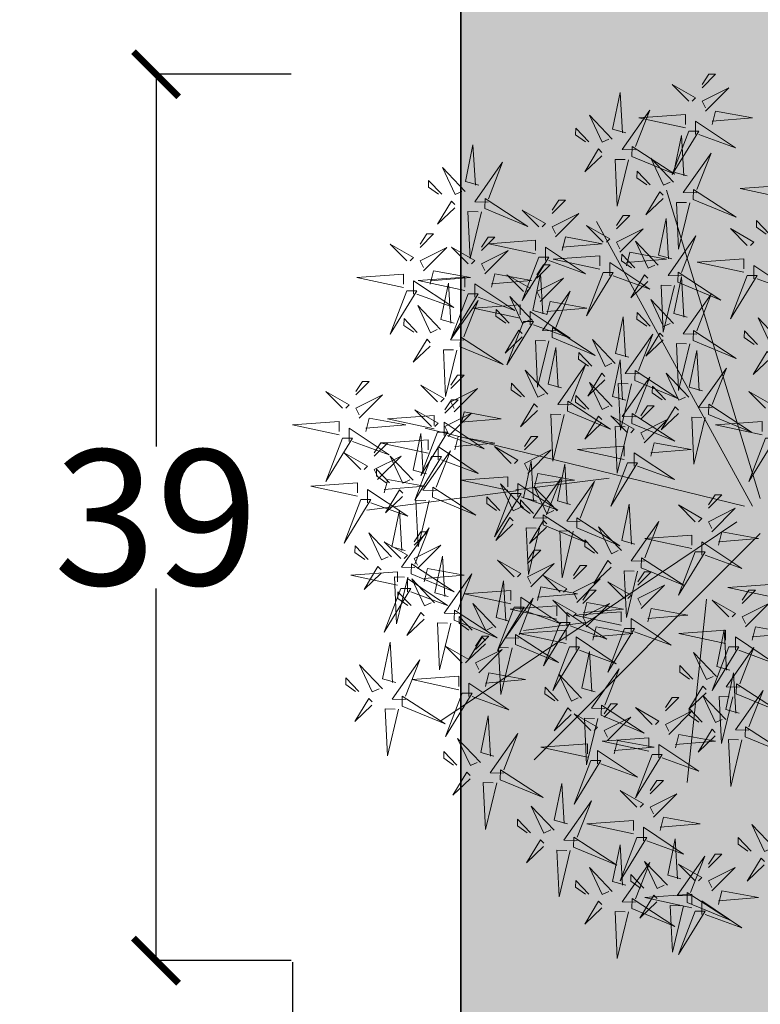
# Model space of a CAD drawing. Units: inches. Extents: x 1704 to 6393, y -157 to 1172.
# Tile 15 of 122: x 1879 to 1912, y 157 to 201. Entities that reach past the tile are written whole.
import ezdxf

# ---------------------------------------------------------------- set-up
doc = ezdxf.new("R2010")
doc.units = ezdxf.units.IN
doc.header["$MEASUREMENT"] = 0
for name, color, linetype, lineweight in [('A-ANNO-DIMS', 7, 'Continuous', 13), ('C-PROP', 7, 'Continuous', 35), ('L-shrub', 74, 'Continuous', 18)]:
    doc.layers.add(name, color=color, linetype=linetype, lineweight=lineweight)
doc.layers.add('L-PLNT-PATT', color=253, linetype='Continuous', lineweight=13, true_color=0x9abc8f)
doc.styles.get("Standard").update_dxf_attribs({"font": 'arial.ttf'})
doc.dimstyles.get("Standard").update_dxf_attribs({"dimtxt": 6, "dimasz": 2, "dimexe": 0.18, "dimexo": 0.0625, "dimgap": 0.09, "dimtad": 0, "dimtih": 1, "dimtoh": 1, "dimdec": 1, "dimzin": 0, "dimdsep": 46, "dimlunit": 3, "dimtxsty": 'Standard', "dimblk": 'ARCHTICK', "dimcen": 0.09, "dimadec": 0, "dimazin": 0, "dimtfac": 1, "dimtdec": 1, "dimtofl": 0, "dimtmove": 0, "dimatfit": 3, "dimfxl": 1, "dimtolj": 1, "dimtzin": 0, "dimarcsym": 0})

# ---------------------------------------------------------------- blocks, each defined once
blk = doc.blocks.new('shrub3')
for p, q in [((-11.38, -5.19), (-224.23, -69.78)), ((12.87, -5.19), (169.14, -161.27)), ((-5.99, -10.57), (-202.68, -118.21)), ((-5.99, -15.96), (-59.88, -236.62)), ((4.78, -21.34), (142.19, -225.85)), ((58.17, -42.16), (184.8, -55.61)), ((-17.27, -174.02), (-25.36, -109.43)), ((74.33, -125.58), (79.72, -168.64)), ((-16.77, -172.03), (-3.3, -276.98))]:
    blk.add_line(p, q)
for points in [[(-163.04, -9.56), (-172.27, -9.56), (-153.8, 18.11), (-163.04, -7.25)], [(86.56, -10.73), (77.32, -8.43), (81.94, 16.94), (84.25, -10.73)], [(153.14, -15.45), (165.42, 14.26), (146.23, -15.28), (153.14, -15.45)], [(-218.53, 13.17), (-225.46, -19.11), (-227.77, 13.17), (-220.84, 13.17)], [(-119.49, 9.1), (-136.03, -6.65), (-117.36, 2.12), (-119.55, 6.79)], [(123.46, -21.81), (135.74, 7.91), (116.55, -21.63), (123.46, -21.81)], [(-193.91, 1.36), (-203.36, -7.64), (-198.75, -7.76), (-193.97, -0.95)], [(-108.14, 1.89), (-96.9, -9.94), (-112.81, -0.3), (-110.44, 1.95)], [(-73.76, -1.46), (-85.3, -12.99), (-76.07, 3.15), (-73.76, 0.84)], [(-52.98, -1.46), (-22.97, -12.99), (-52.98, 5.45), (-52.98, -1.46)], [(57.07, 4.7), (50.14, -27.58), (47.83, 4.7), (54.76, 4.7)], [(77.32, -15.34), (61.16, 0.8), (70.4, -17.65), (75.02, -15.34)], [(93.49, -22.26), (84.25, -22.26), (102.72, 5.41), (93.49, -19.96)], [(230.31, 4.87), (213.77, -10.89), (232.44, -2.12), (230.25, 2.56)], [(-55.29, -3.77), (-62.22, -36.05), (-64.53, -3.77), (-57.6, -3.77)], [(20.84, -34.02), (11.6, -31.72), (16.22, -6.36), (18.53, -34.02)], [(148.59, -13.03), (148.36, -22.26), (121.16, -3.11), (146.29, -12.97)], [(241.66, -2.35), (252.9, -14.18), (237, -4.54), (239.36, -2.29)], [(268.88, -34.02), (259.65, -31.72), (264.26, -6.36), (266.57, -34.02)], [(-269.6, -38.26), (-278.84, -35.95), (-274.22, -10.59), (-271.91, -38.26)], [(-186.12, -14.17), (-197.67, -25.7), (-188.43, -9.56), (-186.12, -11.86)], [(-165.34, -14.17), (-135.33, -25.7), (-165.34, -7.25), (-165.34, -14.17)], [(-117.59, -7.11), (-127.04, -16.11), (-122.43, -16.23), (-117.65, -9.42)], [(-69.46, -40.86), (-57.18, -11.15), (-76.37, -40.69), (-69.46, -40.86)], [(61.16, -17.65), (51.93, -8.43), (51.93, -13.04), (58.86, -17.65)], [(118.91, -19.38), (118.68, -28.61), (91.48, -9.46), (116.61, -19.33)], [(232.21, -11.35), (222.76, -20.35), (227.37, -20.46), (232.16, -13.66)], [(-167.65, -16.47), (-174.58, -48.76), (-176.89, -16.47), (-169.96, -16.47)], [(27.76, -45.55), (18.53, -45.55), (37, -17.88), (27.76, -43.25)], [(91.18, -26.87), (121.19, -38.4), (91.18, -19.96), (91.18, -26.87)], [(136.89, -19.67), (134.36, -28.84), (109.12, -23.59), (136.84, -21.97)], [(155.39, -17.82), (187.49, -25.55), (155.16, -27.05), (155.33, -20.13)], [(275.81, -45.55), (266.57, -45.55), (285.04, -17.88), (275.81, -43.25)], [(-278.84, -42.87), (-295, -26.73), (-285.76, -45.18), (-281.15, -42.87)], [(-262.68, -49.79), (-271.91, -49.79), (-253.44, -22.12), (-262.68, -47.48)], [(-217.86, -51.45), (-205.58, -21.74), (-224.77, -51.28), (-217.86, -51.45)], [(-120.34, -51.45), (-108.06, -21.74), (-127.25, -51.28), (-120.34, -51.45)], [(11.6, -38.64), (-4.56, -22.5), (4.68, -40.94), (9.3, -38.64)], [(70.4, -26.87), (58.86, -38.4), (68.09, -22.26), (70.4, -24.57)], [(107.21, -26.02), (104.68, -35.19), (79.44, -29.94), (107.16, -28.33)], [(125.71, -24.17), (157.81, -31.9), (125.48, -33.4), (125.65, -26.48)], [(259.65, -38.64), (243.49, -22.5), (252.72, -40.94), (257.34, -38.64)], [(267.62, -55.68), (279.9, -25.97), (260.71, -55.51), (267.62, -55.68)], [(-160.62, -62.04), (-148.34, -32.32), (-167.53, -61.86), (-160.62, -62.04)], [(-74.01, -38.44), (-74.24, -47.67), (-101.44, -28.52), (-76.31, -38.38)], [(-4.56, -40.94), (-13.79, -31.72), (-13.79, -36.33), (-6.86, -40.94)], [(88.87, -29.18), (81.94, -61.46), (79.63, -29.18), (86.56, -29.18)], [(141.27, -29.01), (124.73, -44.76), (143.4, -35.99), (141.21, -31.32)], [(243.49, -40.94), (234.25, -31.72), (234.25, -36.33), (241.18, -40.94)], [(-295, -45.18), (-304.23, -35.95), (-304.23, -40.56), (-297.31, -45.18)], [(-222.41, -49.03), (-222.64, -58.26), (-249.84, -39.1), (-224.72, -48.97)], [(-124.89, -49.03), (-125.12, -58.26), (-152.32, -39.1), (-127.2, -48.97)], [(111.59, -35.37), (95.05, -51.12), (113.72, -42.35), (111.53, -37.67)], [(152.62, -36.23), (163.86, -48.05), (147.96, -38.42), (150.32, -36.17)], [(160.76, -63.67), (151.53, -61.36), (156.14, -36), (158.45, -63.67)], [(-264.99, -54.4), (-234.97, -65.93), (-264.99, -47.48), (-264.99, -54.4)], [(-85.71, -45.07), (-88.24, -54.25), (-113.48, -49), (-85.77, -47.38)], [(-67.21, -43.23), (-35.11, -50.96), (-67.44, -52.46), (-67.27, -45.54)], [(4.68, -50.16), (-6.86, -61.69), (2.37, -45.55), (4.68, -47.86)], [(25.46, -50.16), (55.47, -61.69), (25.46, -43.25), (25.46, -50.16)], [(122.94, -42.58), (134.18, -54.41), (118.28, -44.77), (120.64, -42.52)], [(143.17, -45.23), (133.72, -54.23), (138.33, -54.34), (143.12, -47.53)], [(167.69, -75.2), (158.45, -75.2), (176.92, -47.53), (167.69, -72.89)], [(218, -74.25), (208.77, -71.95), (213.38, -46.59), (215.69, -74.25)], [(263.07, -53.26), (262.84, -62.49), (235.64, -43.34), (260.77, -53.2)], [(252.72, -50.16), (241.18, -61.69), (250.41, -45.55), (252.72, -47.86)], [(273.5, -50.16), (303.51, -61.69), (273.5, -43.25), (273.5, -50.16)], [(-285.76, -54.4), (-297.31, -65.93), (-288.07, -49.79), (-285.76, -52.09)], [(-215.61, -53.82), (-183.51, -61.55), (-215.84, -63.05), (-215.67, -56.12)], [(-165.17, -59.61), (-165.4, -68.85), (-192.6, -49.69), (-167.48, -59.56)], [(-118.09, -53.82), (-85.99, -61.55), (-118.32, -63.05), (-118.15, -56.12)], [(-40.64, -80.61), (-49.88, -78.3), (-45.26, -52.94), (-42.95, -80.61)], [(23.15, -52.47), (16.22, -84.75), (13.91, -52.47), (20.84, -52.47)], [(113.49, -51.58), (104.04, -60.58), (108.65, -60.69), (113.43, -53.89)], [(151.53, -68.28), (135.37, -52.14), (144.6, -70.59), (149.22, -68.28)], [(271.19, -52.47), (264.26, -84.75), (261.95, -52.47), (268.88, -52.47)], [(-267.29, -56.71), (-274.22, -88.99), (-276.53, -56.71), (-269.6, -56.71)], [(-234.11, -55.66), (-236.65, -64.84), (-261.89, -59.59), (-234.17, -57.97)], [(-136.59, -55.66), (-139.12, -64.84), (-164.36, -59.59), (-136.65, -57.97)], [(-81.33, -54.42), (-97.87, -70.17), (-79.2, -61.4), (-81.39, -56.73)], [(36.54, -87.45), (48.82, -57.73), (29.63, -87.27), (36.54, -87.45)], [(73.84, -82.72), (64.6, -80.42), (69.22, -55.06), (71.53, -82.72)], [(224.93, -85.78), (215.69, -85.78), (234.16, -58.11), (224.93, -83.48)], [(251.37, -59.9), (248.84, -69.07), (223.6, -63.82), (251.32, -62.2)], [(269.87, -58.05), (301.97, -65.78), (269.64, -67.28), (269.81, -60.36)], [(-247.54, -93.8), (-235.26, -64.08), (-254.45, -93.62), (-247.54, -93.8)], [(-229.73, -65.01), (-246.27, -80.76), (-227.6, -71.99), (-229.79, -67.32)], [(-176.87, -66.25), (-179.4, -75.42), (-204.64, -70.17), (-176.93, -68.56)], [(-158.37, -64.4), (-126.27, -72.13), (-158.6, -73.63), (-158.43, -66.71)], [(-132.21, -65.01), (-148.75, -80.76), (-130.08, -71.99), (-132.27, -67.32)], [(-92.78, -91.68), (-80.5, -61.97), (-99.69, -91.51), (-92.78, -91.68)], [(-69.98, -61.63), (-58.74, -73.46), (-74.65, -63.83), (-72.28, -61.58)], [(-63.1, -93.8), (-50.82, -64.08), (-70.01, -93.62), (-63.1, -93.8)], [(-33.72, -92.14), (-42.95, -92.14), (-24.48, -64.47), (-33.72, -89.83)], [(80.77, -94.25), (71.53, -94.25), (90, -66.58), (80.77, -91.95)], [(135.37, -70.59), (126.13, -61.36), (126.13, -65.97), (133.06, -70.59)], [(208.77, -78.87), (192.61, -62.73), (201.84, -81.17), (206.46, -78.87)], [(271.86, -93.8), (284.14, -64.08), (264.95, -93.62), (271.86, -93.8)], [(-218.38, -72.22), (-207.14, -84.05), (-223.05, -74.41), (-220.68, -72.16)], [(-172.08, -97.55), (-181.32, -95.24), (-176.7, -69.88), (-174.39, -97.55)], [(-120.86, -72.22), (-109.62, -84.05), (-125.53, -74.41), (-123.16, -72.16)], [(-79.43, -70.63), (-88.88, -79.64), (-84.27, -79.75), (-79.49, -72.94)], [(-49.88, -85.22), (-66.04, -69.08), (-56.8, -87.52), (-52.18, -85.22)], [(64.6, -87.34), (48.44, -71.2), (57.68, -89.64), (62.3, -87.34)], [(165.38, -79.81), (195.39, -91.34), (165.38, -72.89), (165.38, -79.81)], [(192.61, -81.17), (183.37, -71.95), (183.37, -76.56), (190.3, -81.17)], [(255.75, -69.24), (239.21, -85), (257.88, -76.23), (255.7, -71.55)], [(-252.09, -91.37), (-252.32, -100.61), (-279.52, -81.45), (-254.4, -91.32)], [(-227.83, -81.22), (-237.28, -90.22), (-232.67, -90.34), (-227.89, -83.53)], [(-172.49, -75.6), (-189.03, -91.35), (-170.36, -82.58), (-172.55, -77.9)], [(-165.16, -109.08), (-174.39, -109.08), (-155.92, -81.41), (-165.16, -106.77)], [(-130.31, -81.22), (-139.76, -90.22), (-135.15, -90.34), (-130.37, -83.53)], [(-97.33, -89.26), (-97.56, -98.49), (-124.76, -79.33), (-99.63, -89.2)], [(-67.65, -91.37), (-67.88, -100.61), (-95.08, -81.45), (-69.95, -91.32)], [(-66.04, -87.52), (-75.27, -78.3), (-75.27, -82.91), (-68.34, -87.52)], [(31.99, -85.02), (31.76, -94.25), (4.56, -75.1), (29.69, -84.96)], [(48.44, -89.64), (39.21, -80.42), (39.21, -85.03), (46.14, -89.64)], [(144.6, -79.81), (133.06, -91.34), (142.29, -75.2), (144.6, -77.5)], [(165, -106.02), (155.77, -103.71), (160.38, -78.35), (162.69, -106.02)], [(267.31, -91.37), (267.08, -100.61), (239.88, -81.45), (265.01, -91.32)], [(267.1, -76.46), (278.34, -88.28), (262.44, -78.65), (264.8, -76.4)], [(-181.32, -102.16), (-197.48, -86.02), (-188.24, -104.46), (-183.63, -102.16)], [(-161.14, -82.81), (-149.9, -94.64), (-165.81, -85), (-163.44, -82.75)], [(138.3, -114.97), (150.58, -85.26), (131.39, -114.8), (138.3, -114.97)], [(163.07, -82.11), (156.14, -114.39), (153.83, -82.11), (160.76, -82.11)], [(201.84, -90.4), (190.3, -101.92), (199.53, -85.78), (201.84, -88.09)], [(222.62, -90.4), (252.63, -101.92), (222.62, -83.48), (222.62, -90.4)], [(257.65, -85.46), (248.2, -94.46), (252.81, -94.57), (257.6, -87.76)], [(-170.59, -91.81), (-180.04, -100.81), (-175.43, -100.93), (-170.65, -94.12)], [(-90.53, -94.05), (-58.43, -101.78), (-90.76, -103.28), (-90.59, -96.35)], [(-56.8, -96.75), (-68.34, -108.28), (-59.11, -92.14), (-56.8, -94.44)], [(-36.02, -96.75), (-6.01, -108.28), (-36.02, -89.83), (-36.02, -96.75)], [(20.29, -91.66), (17.76, -100.83), (-7.48, -95.58), (20.23, -93.97)], [(38.79, -89.81), (70.89, -97.54), (38.56, -99.04), (38.73, -92.12)], [(57.68, -98.86), (46.14, -110.39), (55.37, -94.25), (57.68, -96.56)], [(86.56, -120.84), (77.32, -118.53), (81.94, -93.17), (84.25, -120.84)], [(78.46, -98.86), (108.47, -110.39), (78.46, -91.95), (78.46, -98.86)], [(155.77, -110.63), (139.61, -94.49), (148.84, -112.93), (153.46, -110.63)], [(171.93, -117.54), (162.69, -117.54), (181.16, -89.88), (171.93, -115.24)], [(220.31, -92.7), (213.38, -124.98), (211.07, -92.7), (218, -92.7)], [(-263.79, -98.01), (-266.33, -107.18), (-291.57, -101.93), (-263.85, -100.32)], [(-245.29, -96.16), (-213.19, -103.89), (-245.52, -105.4), (-245.35, -98.47)], [(-197.48, -104.46), (-206.71, -95.24), (-206.71, -99.85), (-199.79, -104.46)], [(-109.03, -95.89), (-111.56, -105.07), (-136.8, -99.82), (-109.09, -98.2)], [(-79.35, -98.01), (-81.88, -107.18), (-107.12, -101.93), (-79.41, -100.32)], [(-60.85, -96.16), (-28.75, -103.89), (-61.08, -105.4), (-60.91, -98.47)], [(-38.33, -99.05), (-45.26, -131.33), (-47.57, -99.05), (-40.64, -99.05)], [(24.67, -101), (8.13, -116.76), (26.8, -107.99), (24.61, -103.31)], [(69.6, -127.19), (60.36, -124.88), (64.98, -99.52), (67.29, -127.19)], [(76.15, -101.17), (69.22, -133.45), (66.91, -101.17), (73.84, -101.17)], [(255.61, -98.01), (253.08, -107.18), (227.84, -101.93), (255.56, -100.32)], [(274.11, -96.16), (306.21, -103.89), (273.88, -105.4), (274.05, -98.47)], [(-259.41, -107.36), (-275.95, -123.11), (-257.28, -114.34), (-259.47, -109.66)], [(-167.46, -113.69), (-137.45, -125.22), (-167.46, -106.77), (-167.46, -113.69)], [(-104.65, -105.24), (-121.19, -120.99), (-102.52, -112.22), (-104.71, -107.55)], [(-74.97, -107.36), (-91.51, -123.11), (-72.84, -114.34), (-75.03, -109.66)], [(-71.58, -138.26), (-59.3, -108.55), (-78.49, -138.09), (-71.58, -138.26)], [(8.98, -131.91), (21.26, -102.2), (2.07, -131.74), (8.98, -131.91)], [(36.02, -108.22), (47.26, -120.04), (31.36, -110.41), (33.72, -108.16)], [(93.49, -132.37), (84.25, -132.37), (102.72, -104.7), (93.49, -130.06)], [(133.75, -112.55), (133.52, -121.78), (106.32, -102.62), (131.45, -112.49)], [(139.61, -112.93), (130.37, -103.71), (130.37, -108.32), (137.3, -112.93)], [(229.46, -134.03), (241.74, -104.31), (222.55, -133.86), (229.46, -134.03)], [(259.99, -107.36), (243.45, -123.11), (262.12, -114.34), (259.94, -109.66)], [(-248.06, -114.57), (-236.82, -126.4), (-252.73, -116.76), (-250.36, -114.51)], [(-188.24, -113.69), (-199.79, -125.22), (-190.55, -109.08), (-188.24, -111.38)], [(-182.68, -142.01), (-191.92, -139.71), (-187.3, -114.34), (-184.99, -142.01)], [(-93.3, -112.45), (-82.06, -124.28), (-97.97, -114.64), (-95.6, -112.39)], [(-63.62, -114.57), (-52.38, -126.4), (-68.29, -116.76), (-65.92, -114.51)], [(77.32, -125.45), (61.16, -109.31), (70.4, -127.75), (75.02, -125.45)], [(76.53, -138.72), (67.29, -138.72), (85.76, -111.05), (76.53, -136.41)], [(169.62, -122.16), (199.63, -133.69), (169.62, -115.24), (169.62, -122.16)], [(271.34, -114.57), (282.58, -126.4), (266.68, -116.76), (269.04, -114.51)], [(-169.77, -115.99), (-176.7, -148.27), (-179.01, -115.99), (-172.08, -115.99)], [(-122.46, -148.85), (-110.18, -119.14), (-129.37, -148.68), (-122.46, -148.85)], [(-102.75, -121.45), (-112.2, -130.45), (-107.59, -130.57), (-102.81, -123.76)], [(4.43, -129.49), (4.2, -138.72), (-23, -119.56), (2.13, -129.43)], [(26.57, -117.22), (17.12, -126.22), (21.73, -126.33), (26.51, -119.53)], [(60.36, -131.8), (44.2, -115.66), (53.44, -134.11), (58.06, -131.8)], [(61.16, -127.75), (51.93, -118.53), (51.93, -123.14), (58.86, -127.75)], [(122.05, -119.18), (119.52, -128.36), (94.28, -123.11), (122, -121.49)], [(148.84, -122.16), (137.3, -133.69), (146.53, -117.54), (148.84, -119.85)], [(140.55, -117.34), (172.65, -125.07), (140.32, -126.57), (140.49, -119.65)], [(224.91, -131.61), (224.68, -140.84), (197.48, -121.68), (222.61, -131.55)], [(-257.51, -123.57), (-266.96, -132.57), (-262.35, -132.69), (-257.57, -125.88)], [(-175.76, -153.54), (-184.99, -153.54), (-166.52, -125.87), (-175.76, -151.23)], [(-138.16, -152.6), (-147.4, -150.29), (-142.78, -124.93), (-140.47, -152.6)], [(-76.13, -135.84), (-76.36, -145.07), (-103.56, -125.92), (-78.43, -135.78)], [(-73.07, -123.57), (-82.52, -132.57), (-77.91, -132.69), (-73.13, -125.88)], [(6.86, -155.2), (19.14, -125.49), (-0.05, -155.03), (6.86, -155.2)], [(44.2, -134.11), (34.97, -124.88), (34.97, -129.5), (41.9, -134.11)], [(126.43, -128.53), (109.89, -144.28), (128.56, -135.51), (126.37, -130.84)], [(167.31, -124.46), (160.38, -156.74), (158.07, -124.46), (165, -124.46)], [(261.89, -123.57), (252.44, -132.57), (257.05, -132.69), (261.84, -125.88)], [(-191.92, -146.62), (-208.08, -130.48), (-198.84, -148.93), (-194.23, -146.62)], [(-19.44, -161.07), (-28.68, -158.76), (-24.06, -133.4), (-21.75, -161.07)], [(11.23, -134.28), (43.33, -142.01), (11, -143.51), (11.17, -136.58)], [(59, -158.95), (49.76, -156.64), (54.38, -131.28), (56.69, -158.95)], [(70.4, -136.98), (58.86, -148.51), (68.09, -132.37), (70.4, -134.67)], [(91.18, -136.98), (121.19, -148.51), (91.18, -130.06), (91.18, -136.98)], [(137.78, -135.74), (149.02, -147.57), (133.12, -137.94), (135.48, -135.69)], [(-208.08, -148.93), (-217.31, -139.71), (-217.31, -144.32), (-210.39, -148.93)], [(-147.4, -157.21), (-163.56, -141.07), (-154.32, -159.52), (-149.71, -157.21)], [(-127.01, -146.43), (-127.24, -155.66), (-154.44, -136.5), (-129.32, -146.37)], [(-131.24, -164.13), (-140.47, -164.13), (-122, -136.46), (-131.24, -161.82)], [(-87.83, -142.48), (-90.36, -151.65), (-115.6, -146.4), (-87.89, -144.78)], [(-69.33, -140.63), (-37.23, -148.36), (-69.56, -149.86), (-69.39, -142.94)], [(-7.27, -136.12), (-9.8, -145.3), (-35.04, -140.05), (-7.33, -138.43)], [(53.44, -143.33), (41.9, -154.86), (51.13, -138.72), (53.44, -141.02)], [(74.22, -143.33), (104.23, -154.86), (74.22, -136.41), (74.22, -143.33)], [(88.87, -139.28), (81.94, -171.56), (79.63, -139.28), (86.56, -139.28)], [(213.21, -138.24), (210.68, -147.41), (185.44, -142.16), (213.16, -140.55)], [(231.71, -136.39), (263.81, -144.13), (231.48, -145.63), (231.65, -138.7)], [(-28.68, -165.68), (-44.84, -149.54), (-35.6, -167.99), (-30.98, -165.68)], [(2.31, -152.78), (2.08, -162.01), (-25.12, -142.86), (0.01, -152.72)], [(-12.52, -172.6), (-21.75, -172.6), (-3.28, -144.93), (-12.52, -170.29)], [(-2.89, -145.47), (-19.43, -161.22), (-0.76, -152.45), (-2.95, -147.78)], [(49.76, -163.56), (33.6, -147.42), (42.84, -165.87), (47.46, -163.56)], [(65.93, -170.48), (56.69, -170.48), (75.16, -142.81), (65.93, -168.17)], [(71.91, -145.64), (64.98, -177.92), (62.67, -145.64), (69.6, -145.64)], [(89.54, -174.26), (101.82, -144.54), (82.63, -174.09), (89.54, -174.26)], [(128.33, -144.74), (118.88, -153.74), (123.49, -153.86), (128.27, -147.05)], [(217.59, -147.59), (201.05, -163.34), (219.72, -154.57), (217.53, -149.9)], [(-198.84, -158.15), (-210.39, -169.68), (-201.15, -153.54), (-198.84, -155.85)], [(-178.06, -158.15), (-148.05, -169.68), (-178.06, -151.23), (-178.06, -158.15)], [(-163.56, -159.52), (-172.79, -150.29), (-172.79, -154.9), (-165.87, -159.52)], [(-138.71, -153.06), (-141.24, -162.24), (-166.48, -156.99), (-138.77, -155.37)], [(-120.21, -151.22), (-88.11, -158.95), (-120.44, -160.45), (-120.27, -153.52)], [(-83.45, -151.82), (-99.99, -167.57), (-81.32, -158.8), (-83.51, -154.13)], [(8.46, -152.68), (19.7, -164.51), (3.8, -154.87), (6.16, -152.62)], [(182.82, -184.85), (195.1, -155.13), (175.91, -184.67), (182.82, -184.85)], [(228.94, -154.8), (240.18, -166.63), (224.28, -156.99), (226.64, -154.74)], [(-180.37, -160.46), (-187.3, -192.74), (-189.61, -160.46), (-182.68, -160.46)], [(-157.24, -190.71), (-166.48, -188.41), (-161.86, -163.04), (-159.55, -190.71)], [(-134.33, -162.41), (-150.87, -178.16), (-132.2, -169.39), (-134.39, -164.72)], [(-133.54, -168.74), (-103.53, -180.27), (-133.54, -161.82), (-133.54, -168.74)], [(-72.1, -159.03), (-60.86, -170.86), (-76.77, -161.23), (-74.4, -158.98)], [(-44.84, -167.99), (-54.07, -158.76), (-54.07, -163.37), (-47.14, -167.99)], [(-9.39, -159.41), (-11.92, -168.59), (-37.16, -163.34), (-9.45, -161.72)], [(-0.99, -161.68), (-10.44, -170.68), (-5.83, -170.8), (-1.05, -163.99)], [(9.11, -157.57), (41.21, -165.3), (8.88, -166.8), (9.05, -159.88)], [(33.6, -165.87), (24.37, -156.64), (24.37, -161.26), (31.3, -165.87)], [(84.99, -171.84), (84.76, -181.07), (57.56, -161.91), (82.69, -171.78)], [(-211.5, -195.43), (-199.22, -165.72), (-218.41, -195.26), (-211.5, -195.43)], [(-154.32, -168.74), (-165.87, -180.27), (-156.63, -164.13), (-154.32, -166.43)], [(-122.98, -169.62), (-111.74, -181.45), (-127.65, -171.81), (-125.28, -169.56)], [(-81.55, -168.04), (-91, -177.04), (-86.39, -177.15), (-81.61, -170.34)], [(-5.01, -168.76), (-21.55, -184.51), (-2.88, -175.74), (-5.07, -171.07)], [(63.62, -175.09), (93.63, -186.62), (63.62, -168.17), (63.62, -175.09)], [(118.36, -194.95), (109.13, -192.64), (113.74, -167.28), (116.05, -194.95)], [(219.49, -163.8), (210.04, -172.8), (214.65, -172.92), (219.44, -166.11)], [(-150.32, -202.24), (-159.55, -202.24), (-141.08, -174.57), (-150.32, -199.93)], [(-135.85, -171.04), (-142.78, -203.33), (-145.09, -171.04), (-138.16, -171.04)], [(-35.6, -177.21), (-47.14, -188.74), (-37.91, -172.6), (-35.6, -174.9)], [(-14.82, -177.21), (15.19, -188.74), (-14.82, -170.29), (-14.82, -177.21)], [(6.34, -175.97), (17.58, -187.8), (1.68, -178.17), (4.04, -175.92)], [(42.84, -175.09), (31.3, -186.62), (40.53, -170.48), (42.84, -172.79)], [(91.79, -176.62), (123.89, -184.36), (91.56, -185.86), (91.73, -178.93)], [(178.27, -182.42), (178.04, -191.65), (150.84, -172.5), (175.97, -182.36)], [(-216.05, -193.01), (-216.28, -202.24), (-243.48, -183.09), (-218.36, -192.95)], [(-166.48, -195.32), (-182.64, -179.18), (-173.4, -197.63), (-168.79, -195.32)], [(-132.43, -178.62), (-141.88, -187.62), (-137.27, -187.74), (-132.49, -180.93)], [(-116.1, -212.37), (-103.82, -182.66), (-123.01, -212.2), (-116.1, -212.37)], [(-17.13, -179.51), (-24.06, -211.79), (-26.37, -179.51), (-19.44, -179.51)], [(73.29, -178.47), (70.76, -187.64), (45.52, -182.39), (73.23, -180.78)], [(61.31, -177.4), (54.38, -209.68), (52.07, -177.4), (59, -177.4)], [(109.13, -199.56), (92.96, -183.42), (102.2, -201.86), (106.82, -199.56)], [(125.29, -206.48), (116.05, -206.48), (134.52, -178.81), (125.29, -204.17)], [(-182.64, -197.63), (-191.87, -188.41), (-191.87, -193.02), (-184.95, -197.63)], [(-61.84, -211.89), (-71.08, -209.58), (-66.46, -184.22), (-64.15, -211.89)], [(-44.88, -216.12), (-54.12, -213.81), (-49.5, -188.45), (-47.19, -216.12)], [(-3.11, -184.97), (-12.56, -193.97), (-7.95, -194.09), (-3.17, -187.28)], [(77.67, -187.82), (61.13, -203.57), (79.8, -194.8), (77.61, -190.13)], [(72.58, -216.61), (84.86, -186.89), (65.67, -216.43), (72.58, -216.61)], [(166.57, -189.06), (164.04, -198.23), (138.8, -192.98), (166.52, -191.37)], [(185.07, -187.21), (217.17, -194.94), (184.84, -196.44), (185.01, -189.52)], [(-54.92, -223.41), (-64.15, -223.41), (-45.68, -195.75), (-54.92, -221.11)], [(92.96, -201.86), (83.73, -192.64), (83.73, -197.25), (90.66, -201.86)], [(89.02, -195.03), (100.26, -206.86), (84.36, -197.22), (86.72, -194.97)], [(-227.75, -199.64), (-230.29, -208.82), (-255.53, -203.57), (-227.81, -201.95)], [(-209.25, -197.8), (-177.15, -205.53), (-209.48, -207.03), (-209.31, -200.11)], [(-173.4, -206.85), (-184.95, -218.38), (-175.71, -202.24), (-173.4, -204.55)], [(-152.62, -206.85), (-122.61, -218.38), (-152.62, -199.93), (-152.62, -206.85)], [(-120.65, -209.95), (-120.88, -219.18), (-148.08, -200.02), (-122.96, -209.89)], [(-71.08, -216.5), (-87.24, -200.36), (-78, -218.8), (-73.38, -216.5)], [(-37.96, -227.65), (-47.19, -227.65), (-28.72, -199.98), (-37.96, -225.34)], [(-12.22, -231.43), (0.06, -201.71), (-19.13, -231.26), (-12.22, -231.43)], [(170.95, -198.4), (154.41, -214.16), (173.08, -205.39), (170.89, -200.71)], [(-223.37, -208.99), (-239.91, -224.74), (-221.24, -215.97), (-223.43, -211.3)], [(-159.36, -233.06), (-168.6, -230.75), (-163.98, -205.39), (-161.67, -233.06)], [(-154.93, -209.16), (-161.86, -241.44), (-164.17, -209.16), (-157.24, -209.16)], [(-87.24, -218.8), (-96.47, -209.58), (-96.47, -214.19), (-89.54, -218.8)], [(-54.12, -220.73), (-70.28, -204.59), (-61.04, -223.04), (-56.42, -220.73)], [(46.28, -237.29), (37.04, -234.99), (41.66, -209.63), (43.97, -237.29)], [(68.03, -214.18), (67.8, -223.42), (40.6, -204.26), (65.73, -214.13)], [(79.57, -204.03), (70.12, -213.03), (74.73, -213.15), (79.51, -206.34)], [(102.2, -211.09), (90.66, -222.62), (99.89, -206.48), (102.2, -208.78)], [(122.98, -211.09), (152.99, -222.62), (122.98, -204.17), (122.98, -211.09)], [(182.3, -205.62), (193.54, -217.44), (177.64, -207.81), (180, -205.56)], [(-212.02, -216.2), (-200.78, -228.03), (-216.69, -218.4), (-214.32, -216.15)], [(-152.44, -244.59), (-161.67, -244.59), (-143.2, -216.92), (-152.44, -242.28)], [(-132.35, -216.58), (-134.88, -225.76), (-160.12, -220.51), (-132.41, -218.89)], [(-113.85, -214.74), (-81.75, -222.47), (-114.08, -223.97), (-113.91, -217.05)], [(-70.28, -223.04), (-79.51, -213.81), (-79.51, -218.43), (-72.58, -223.04)], [(40.78, -246.25), (53.06, -216.54), (33.87, -246.08), (40.78, -246.25)], [(120.67, -213.39), (113.74, -245.67), (111.43, -213.39), (118.36, -213.39)], [(172.85, -214.62), (163.4, -223.62), (168.01, -223.73), (172.8, -216.93)], [(-168.6, -237.67), (-184.76, -221.53), (-175.52, -239.98), (-170.91, -237.67)], [(-78, -228.03), (-89.54, -239.55), (-80.31, -223.41), (-78, -225.72)], [(-57.22, -228.03), (-27.21, -239.55), (-57.22, -221.11), (-57.22, -228.03)], [(-16.77, -229.01), (-17, -238.24), (-44.2, -219.08), (-19.07, -228.95)], [(56.33, -220.82), (53.8, -229.99), (28.56, -224.74), (56.27, -223.13)], [(53.21, -248.82), (43.97, -248.82), (62.44, -221.15), (53.21, -246.52)], [(74.83, -218.97), (106.93, -226.7), (74.6, -228.2), (74.77, -221.28)], [(131.94, -252.6), (144.22, -222.89), (125.03, -252.43), (131.94, -252.6)], [(-221.47, -225.2), (-230.92, -234.21), (-226.31, -234.32), (-221.53, -227.51)], [(-184.76, -239.98), (-193.99, -230.75), (-193.99, -235.37), (-187.07, -239.98)], [(-127.97, -225.93), (-144.51, -241.68), (-125.84, -232.91), (-128.03, -228.24)], [(-61.04, -232.26), (-72.58, -243.79), (-63.35, -227.65), (-61.04, -229.95)], [(-59.53, -230.33), (-66.46, -262.61), (-68.77, -230.33), (-61.84, -230.33)], [(-40.26, -232.26), (-10.25, -243.79), (-40.26, -225.34), (-40.26, -232.26)], [(37.04, -241.91), (20.88, -225.77), (30.12, -244.21), (34.74, -241.91)], [(60.71, -230.17), (44.17, -245.92), (62.84, -237.15), (60.65, -232.47)], [(-116.62, -233.14), (-105.38, -244.97), (-121.29, -235.34), (-118.92, -233.09)], [(-28.47, -235.64), (-31, -244.81), (-56.24, -239.56), (-28.53, -237.95)], [(-42.57, -234.57), (-49.5, -266.85), (-51.81, -234.57), (-44.88, -234.57)], [(-15.2, -264.82), (-24.44, -262.51), (-19.82, -237.15), (-17.51, -264.82)], [(-9.97, -233.79), (22.13, -241.53), (-10.2, -243.03), (-10.03, -236.1)], [(36.23, -243.83), (36, -253.06), (8.8, -233.9), (33.93, -243.77)], [(20.88, -244.21), (11.65, -234.99), (11.65, -239.6), (18.58, -244.21)], [(72.06, -237.38), (83.3, -249.21), (67.4, -239.57), (69.76, -237.32)], [(-175.52, -249.2), (-187.07, -260.73), (-177.83, -244.59), (-175.52, -246.89)], [(-154.74, -249.2), (-124.73, -260.73), (-154.74, -242.28), (-154.74, -249.2)], [(-126.07, -242.14), (-135.52, -251.14), (-130.91, -251.26), (-126.13, -244.45)], [(127.39, -250.18), (127.16, -259.41), (99.96, -240.26), (125.09, -250.12)], [(-157.05, -251.51), (-163.98, -283.79), (-166.29, -251.51), (-159.36, -251.51)], [(-57.6, -277.52), (-66.84, -275.22), (-62.22, -249.86), (-59.91, -277.52)], [(-24.09, -244.99), (-40.63, -260.74), (-21.96, -251.97), (-24.15, -247.3)], [(-8.28, -276.35), (-17.51, -276.35), (0.96, -248.68), (-8.28, -274.04)], [(24.53, -250.46), (22, -259.64), (-3.24, -254.39), (24.47, -252.77)], [(30.12, -253.43), (18.58, -264.96), (27.81, -248.82), (30.12, -251.13)], [(43.03, -248.62), (75.13, -256.35), (42.8, -257.85), (42.97, -250.92)], [(50.9, -253.43), (80.91, -264.96), (50.9, -246.52), (50.9, -253.43)], [(62.61, -246.38), (53.16, -255.38), (57.77, -255.49), (62.55, -248.69)], [(-24.44, -269.43), (-40.6, -253.29), (-31.36, -271.74), (-26.74, -269.43)], [(-12.74, -252.2), (-1.5, -264.03), (-17.4, -254.39), (-15.04, -252.14)], [(48.59, -255.74), (41.66, -288.02), (39.35, -255.74), (46.28, -255.74)], [(115.69, -256.81), (113.16, -265.99), (87.92, -260.74), (115.64, -259.12)], [(134.19, -254.97), (166.29, -262.7), (133.96, -264.2), (134.13, -257.28)], [(-50.68, -289.05), (-59.91, -289.05), (-41.44, -261.38), (-50.68, -286.75)], [(-40.6, -271.74), (-49.83, -262.51), (-49.83, -267.13), (-42.9, -271.74)], [(-22.19, -261.2), (-31.64, -270.2), (-27.03, -270.32), (-22.25, -263.51)], [(28.91, -259.81), (12.37, -275.56), (31.04, -266.79), (28.85, -262.12)], [(-66.84, -282.14), (-83, -266), (-73.76, -284.44), (-69.14, -282.14)], [(40.26, -267.02), (51.5, -278.85), (35.6, -269.21), (37.96, -266.96)], [(120.07, -266.16), (103.53, -281.91), (122.2, -273.14), (120.01, -268.47)], [(-83, -284.44), (-92.23, -275.22), (-92.23, -279.83), (-85.3, -284.44)], [(-31.36, -280.96), (-42.9, -292.49), (-33.67, -276.35), (-31.36, -278.65)], [(-10.58, -280.96), (19.43, -292.49), (-10.58, -274.04), (-10.58, -280.96)], [(30.81, -276.02), (21.36, -285.02), (25.97, -285.14), (30.75, -278.33)], [(131.42, -273.37), (142.66, -285.2), (126.76, -275.57), (129.12, -273.32)], [(-12.89, -283.27), (-19.82, -315.55), (-22.13, -283.27), (-15.2, -283.27)], [(121.97, -282.37), (112.52, -291.38), (117.13, -291.49), (121.91, -284.68)], [(-73.76, -293.67), (-85.3, -305.19), (-76.07, -289.05), (-73.76, -291.36)], [(-52.98, -293.67), (-22.97, -305.19), (-52.98, -286.75), (-52.98, -293.67)], [(-55.29, -295.97), (-62.22, -328.25), (-64.53, -295.97), (-57.6, -295.97)]]:
    blk.add_lwpolyline(points)
blk = doc.blocks.new('_ArchTick')
at = {"color": 0, "linetype": 'ByBlock', "const_width": 0.15}
blk.add_lwpolyline([(-0.5, -0.5), (0.5, 0.5)], dxfattribs=at)
blk = doc.blocks.new('*D74')
at = {"layer": 'A-ANNO-DIMS', "color": 0, "lineweight": -2, "transparency": 16777216}
for p, q in [((1890.878, 159.062), (1890.878, 152.884)), ((1931.278, 159.062), (1931.278, 152.884)), ((1890.878, 153.064), (1888.878, 153.064)), ((1931.278, 153.064), (1933.278, 153.064))]:
    blk.add_line(p, q, dxfattribs=at)
at = {"layer": 'Defpoints', "color": 0, "lineweight": -3, "transparency": 16777216}
for p in [(1890.878, 159.124), (1931.278, 159.124), (1931.278, 153.064)]:
    blk.add_point(p, dxfattribs=at)
at = {"layer": 'A-ANNO-DIMS', "color": 0, "lineweight": -2, "transparency": 16777216, "xscale": 2, "yscale": 2, "zscale": 2}
blk.add_blockref('_ArchTick', (1890.878, 153.064), dxfattribs=at)
at = {"layer": 'A-ANNO-DIMS', "color": 0, "lineweight": -2, "transparency": 16777216, "xscale": 2, "yscale": 2, "zscale": 2, "rotation": 180}
blk.add_blockref('_ArchTick', (1931.278, 153.064), dxfattribs=at)
at = {"layer": 'A-ANNO-DIMS', "color": 0, "transparency": 16777216, "insert": (1911.078, 153.064), "char_height": 6, "attachment_point": 5}
blk.add_mtext('\\A1;SHRUB 40', dxfattribs=at)
blk = doc.blocks.new('*D75')
at = {"layer": 'A-ANNO-DIMS', "color": 0, "lineweight": -2, "transparency": 16777216}
for p, q in [((1890.815, 198.475), (1884.637, 198.475)), ((1884.817, 198.475), (1884.817, 181.955)), ((1884.817, 159.124), (1884.817, 175.644)), ((1890.815, 159.124), (1884.637, 159.124))]:
    blk.add_line(p, q, dxfattribs=at)
at = {"layer": 'Defpoints', "color": 0, "lineweight": -3, "transparency": 16777216}
for p in [(1890.878, 198.475), (1884.817, 159.124), (1890.878, 159.124)]:
    blk.add_point(p, dxfattribs=at)
at = {"layer": 'A-ANNO-DIMS', "color": 0, "lineweight": -2, "transparency": 16777216, "xscale": 2, "yscale": 2, "zscale": 2}
for p, rotation in [((1884.817, 198.475), 90), ((1884.817, 159.124), 270)]:
    blk.add_blockref('_ArchTick', p, dxfattribs=dict(at, rotation=rotation))
at = {"layer": 'A-ANNO-DIMS', "color": 0, "transparency": 16777216, "insert": (1884.817, 178.8), "char_height": 6, "attachment_point": 5}
blk.add_mtext('\\A1;39', dxfattribs=at)
blk = doc.blocks.new('*D93')
at = {"layer": 'A-ANNO-DIMS', "color": 0, "lineweight": -2, "transparency": 16777216}
for p, q in [((2605.286, 895.213), (1829.698, 895.213)), ((1829.878, 895.213), (1829.878, 495.866)), ((1829.878, 90.213), (1829.878, 489.56)), ((2605.286, 90.213), (1829.698, 90.213))]:
    blk.add_line(p, q, dxfattribs=at)
at = {"layer": 'Defpoints', "color": 0, "lineweight": -3, "transparency": 16777216}
for p in [(2605.349, 895.213), (1829.878, 90.213), (2605.349, 90.213)]:
    blk.add_point(p, dxfattribs=at)
at = {"layer": 'A-ANNO-DIMS', "color": 0, "lineweight": -2, "transparency": 16777216, "xscale": 2, "yscale": 2, "zscale": 2}
for p, rotation in [((1829.878, 895.213), 90), ((1829.878, 90.213), 270)]:
    blk.add_blockref('_ArchTick', p, dxfattribs=dict(at, rotation=rotation))
at = {"layer": 'A-ANNO-DIMS', "color": 0, "transparency": 16777216, "insert": (1829.878, 492.713), "char_height": 6, "attachment_point": 5}
blk.add_mtext('\\A1;805', dxfattribs=at)

msp = doc.modelspace()

# ---------------------------------------------------------------- hatches: boundary and pattern name
at = {"layer": 'L-PLNT-PATT', "transparency": 33554643}
h = msp.add_hatch(color=256, dxfattribs=at)
h.dxf.hatch_style = 1
h.paths.add_polyline_path([(1975.349, 202.213), (1898.349, 202.213), (1898.349, -3.787), (1975.349, -3.787)])

# ---------------------------------------------------------------- linework, layer by layer
at = {"layer": 'C-PROP'}
msp.add_line((1898.349, -3.787), (1898.349, 1033.213), dxfattribs=at)

# ---------------------------------------------------------------- block references
at = {"layer": 'L-shrub', "xscale": 0.0642956299502212, "yscale": 0.0642956299502212, "zscale": 0.0642956299502212, "rotation": 270}
msp.add_blockref('shrub3', (1911.983, 178.911), dxfattribs=at)

# ---------------------------------------------------------------- dimensions: what is measured, and where the dimension line sits
at = {"layer": 'A-ANNO-DIMS'}
for base, p1, p2, angle, picture, middle in [((1829.878, 90.213), (2605.349, 895.213), (2605.349, 90.213), 90, '*D93', (1829.878, 492.713)), ((1884.817, 159.124), (1890.878, 198.475), (1890.878, 159.124), 270, '*D75', (1884.817, 178.8))]:
    dim = msp.add_linear_dim(base=base, p1=p1, p2=p2, angle=angle, dimstyle='Standard', override={"dimdec": 0, "dimlfac": 1, "dimrnd": 0, "dimzin": 0, "dimdsep": 46, "dimlunit": 2}, dxfattribs=at)
    dim.commit()
    dim.dimension.update_dxf_attribs({"geometry": picture, "text_midpoint": middle})
dim = msp.add_linear_dim(base=(1931.278, 153.064), p1=(1890.878, 159.124), p2=(1931.278, 159.124), text='SHRUB <>', dimstyle='Standard', override={"dimdec": 0, "dimlfac": 1, "dimrnd": 0, "dimzin": 0, "dimdsep": 46, "dimlunit": 2}, dxfattribs=at)
dim.commit()
dim.dimension.update_dxf_attribs({"geometry": '*D74', "text_midpoint": (1911.078, 153.064)})

doc.saveas('drawing.dxf')
